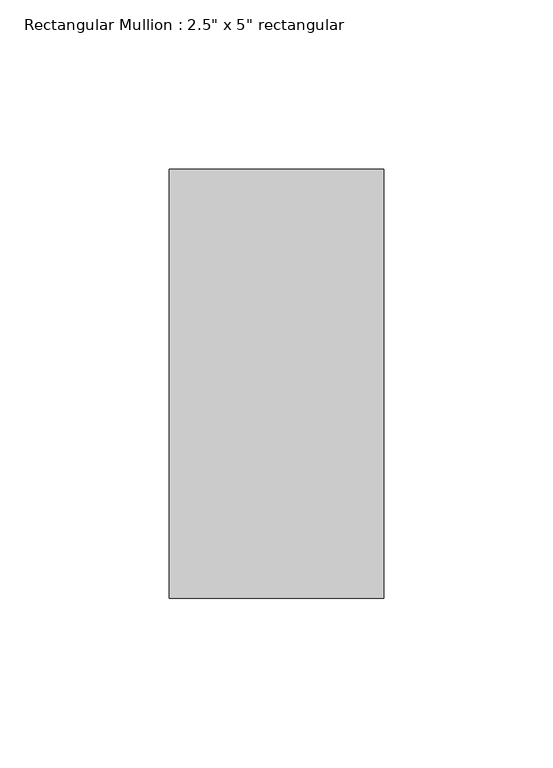
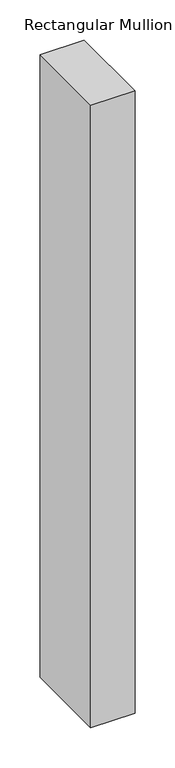
"""IFC4 building model written with IfcOpenShell, lengths in millimetres: member geometry."""

from ifc_helpers import new_model, si_unit, frame, origin, place, context, project, spatial, polyline, outline, extrude, source, transform, mapped, element, save


def member_aead4eab(model_context):
    return source(origin(), model_context, "Body", "SweptSolid", [
        extrude(outline(polyline([(0.0, 63.5), (0.0, -63.5), (-63.5, -63.5), (-63.5, 63.5), (0.0, 63.5)])), frame((0.0, 0.0, -948.3113392), z_axis=(0.0, 0.0, 1.0), x_axis=(1.0, 0.0, 0.0)), (0.0, 0.0, 1.0), 948.3113392),
    ])


if __name__ == "__main__":
    model = new_model("IFC4")
    model_context = context("Model", 3, world=origin())
    ifc_project = project(units=[si_unit("LENGTHUNIT", "METRE", prefix="MILLI")], contexts=[model_context])
    site = spatial("IfcSite", under=ifc_project)
    building = spatial("IfcBuilding", under=site)
    placement = place(None, origin())
    member_shape = member_aead4eab(model_context)
    element("IfcMember", 1, ObjectType="Rectangular Mullion : 2.5\" x 5\" rectangular", at=placement, inside=building, context=model_context, shape_type="MappedRepresentation", body=[
        mapped(member_shape, transform((0.0, 0.0, 0.0), x_axis=(1.0, 0.0, 0.0), y_axis=(0.0, 1.0, 0.0), z_axis=(0.0, 0.0, 1.0))),
    ])
    save(model, "model.ifc")

# Revit data of these elements
# Type "Rectangular Mullion : 2.5\" x 5\" rectangular"
#   built-in parameter 1007304 = 0.416667 (stored number, unit not read)
#   built-in parameter 1007301 = 0.104167 (stored number, unit not read)
#   built-in parameter 1007300 = 0.104167 (stored number, unit not read)
# Element 1 (IfcMember, "Rectangular Mullion : 2.5\" x 5\" rectangular")
#   Materials on its faces: "Aluminum"
# Materials
#   "Aluminum": class "Metal", colour RGB 247 247 247, transparency 0, Description = "Aluminum 6061", Cost = 0
